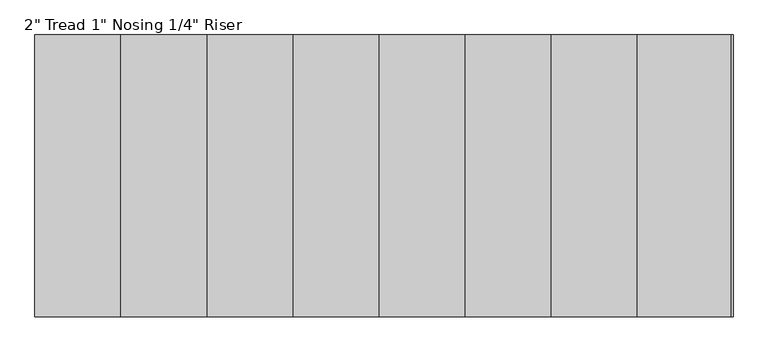
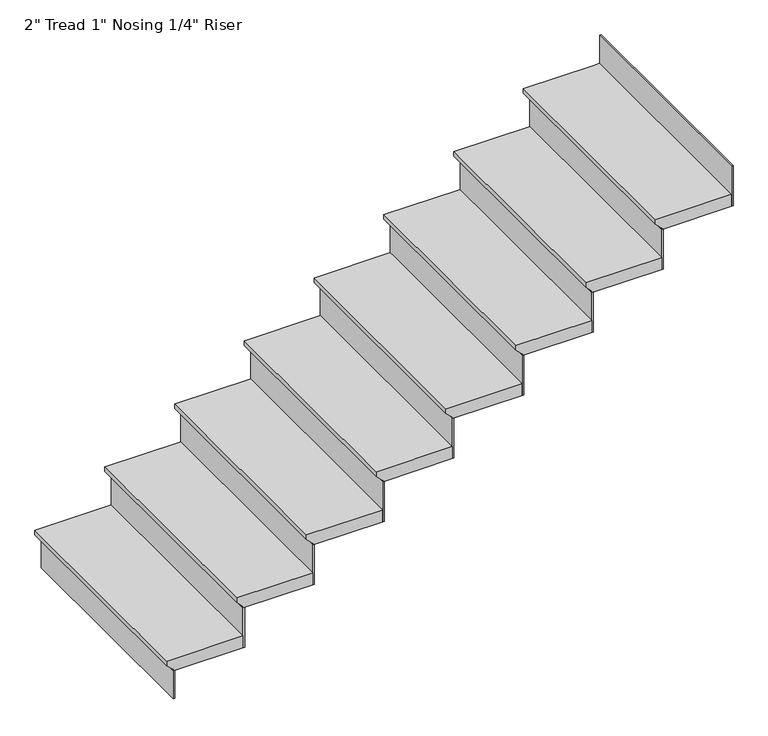
"""IFC4 building model written with IfcOpenShell, lengths in millimetres: stair flight geometry."""

from ifc_helpers import new_model, si_unit, origin, place, context, project, spatial, faceted_brep, source, transform, mapped, element, save


def stair_flight_35773103(model_context):
    return source(origin(), model_context, "Body", "Brep", [
        faceted_brep([(-8529.8389568, 3195.5342758, 150.2833333), (-8529.8389568, 3195.5342758, 169.3333333), (-8529.8389568, 4109.9342758, 169.3333333), (-8529.8389568, 4109.9342758, 150.2833333), (-8504.4389568, 3195.5342758, 124.8833333), (-8504.4389568, 4109.9342758, 124.8833333), (-8225.0389568, 3195.5342758, 169.3333333), (-8225.0389568, 4109.9342758, 169.3333333), (-8504.4389568, 4109.9342758, 118.5333333), (-8225.0389568, 4109.9342758, 118.5333333), (-8225.0389568, 3195.5342758, 118.5333333), (-8504.4389568, 3195.5342758, 118.5333333)], [[[0, 1, 2, 3]], [[4, 0, 3, 5]], [[2, 1, 6, 7]], [[8, 9, 10, 11]], [[2, 7, 9, 8, 5, 3]], [[8, 11, 4, 5]], [[6, 1, 0, 4, 11, 10]], [[7, 6, 10, 9]]]),
        faceted_brep([(-8504.4389568, 3195.5342758, 118.5333333), (-8504.4389568, 3195.5342758, 0.0), (-8498.0889568, 3195.5342758, 0.0), (-8498.0889568, 3195.5342758, 118.5333333), (-8504.4389568, 4109.9342758, 118.5333333), (-8498.0889568, 4109.9342758, 118.5333333), (-8498.0889568, 4109.9342758, 0.0), (-8504.4389568, 4109.9342758, 0.0)], [[[0, 1, 2, 3]], [[4, 5, 6, 7]], [[1, 0, 4, 7]], [[2, 1, 7, 6]], [[3, 2, 6, 5]], [[0, 3, 5, 4]]]),
        faceted_brep([(-8225.0389568, 3195.5342758, 287.8666667), (-8225.0389568, 3195.5342758, 118.5333333), (-8218.6889568, 3195.5342758, 118.5333333), (-8218.6889568, 3195.5342758, 287.8666667), (-8225.0389568, 4109.9342758, 287.8666667), (-8218.6889568, 4109.9342758, 287.8666667), (-8218.6889568, 4109.9342758, 118.5333333), (-8225.0389568, 4109.9342758, 118.5333333)], [[[0, 1, 2, 3]], [[4, 5, 6, 7]], [[1, 0, 4, 7]], [[2, 1, 7, 6]], [[3, 2, 6, 5]], [[0, 3, 5, 4]]]),
        faceted_brep([(-8250.4389568, 4109.9342758, 338.6666667), (-8250.4389568, 3195.5342758, 338.6666667), (-7945.6389568, 3195.5342758, 338.6666667), (-7945.6389568, 4109.9342758, 338.6666667), (-8225.0389568, 4109.9342758, 287.8666667), (-7945.6389568, 4109.9342758, 287.8666667), (-7945.6389568, 3195.5342758, 287.8666667), (-8225.0389568, 3195.5342758, 287.8666667), (-8225.0389568, 4109.9342758, 294.2166667), (-8250.4389568, 4109.9342758, 319.6166667), (-8225.0389568, 3195.5342758, 294.2166667), (-8250.4389568, 3195.5342758, 319.6166667)], [[[0, 1, 2, 3]], [[4, 5, 6, 7]], [[0, 3, 5, 4, 8, 9]], [[4, 7, 10, 8]], [[2, 1, 11, 10, 7, 6]], [[3, 2, 6, 5]], [[11, 1, 0, 9]], [[10, 11, 9, 8]]]),
        faceted_brep([(-7945.6389568, 3195.5342758, 457.2), (-7945.6389568, 3195.5342758, 287.8666667), (-7939.2889568, 3195.5342758, 287.8666667), (-7939.2889568, 3195.5342758, 457.2), (-7945.6389568, 4109.9342758, 457.2), (-7939.2889568, 4109.9342758, 457.2), (-7939.2889568, 4109.9342758, 287.8666667), (-7945.6389568, 4109.9342758, 287.8666667)], [[[0, 1, 2, 3]], [[4, 5, 6, 7]], [[1, 0, 4, 7]], [[2, 1, 7, 6]], [[3, 2, 6, 5]], [[0, 3, 5, 4]]]),
        faceted_brep([(-7971.0389568, 4109.9342758, 508.0), (-7971.0389568, 3195.5342758, 508.0), (-7666.2389568, 3195.5342758, 508.0), (-7666.2389568, 4109.9342758, 508.0), (-7945.6389568, 4109.9342758, 457.2), (-7666.2389568, 4109.9342758, 457.2), (-7666.2389568, 3195.5342758, 457.2), (-7945.6389568, 3195.5342758, 457.2), (-7945.6389568, 4109.9342758, 463.55), (-7971.0389568, 4109.9342758, 488.95), (-7945.6389568, 3195.5342758, 463.55), (-7971.0389568, 3195.5342758, 488.95)], [[[0, 1, 2, 3]], [[4, 5, 6, 7]], [[0, 3, 5, 4, 8, 9]], [[4, 7, 10, 8]], [[2, 1, 11, 10, 7, 6]], [[3, 2, 6, 5]], [[11, 1, 0, 9]], [[10, 11, 9, 8]]]),
        faceted_brep([(-7666.2389568, 3195.5342758, 626.5333333), (-7666.2389568, 3195.5342758, 457.2), (-7659.8889568, 3195.5342758, 457.2), (-7659.8889568, 3195.5342758, 626.5333333), (-7666.2389568, 4109.9342758, 626.5333333), (-7659.8889568, 4109.9342758, 626.5333333), (-7659.8889568, 4109.9342758, 457.2), (-7666.2389568, 4109.9342758, 457.2)], [[[0, 1, 2, 3]], [[4, 5, 6, 7]], [[1, 0, 4, 7]], [[2, 1, 7, 6]], [[3, 2, 6, 5]], [[0, 3, 5, 4]]]),
        faceted_brep([(-7691.6389568, 4109.9342758, 677.3333333), (-7691.6389568, 3195.5342758, 677.3333333), (-7386.8389568, 3195.5342758, 677.3333333), (-7386.8389568, 4109.9342758, 677.3333333), (-7666.2389568, 4109.9342758, 626.5333333), (-7386.8389568, 4109.9342758, 626.5333333), (-7386.8389568, 3195.5342758, 626.5333333), (-7666.2389568, 3195.5342758, 626.5333333), (-7666.2389568, 4109.9342758, 632.8833333), (-7691.6389568, 4109.9342758, 658.2833333), (-7666.2389568, 3195.5342758, 632.8833333), (-7691.6389568, 3195.5342758, 658.2833333)], [[[0, 1, 2, 3]], [[4, 5, 6, 7]], [[0, 3, 5, 4, 8, 9]], [[4, 7, 10, 8]], [[2, 1, 11, 10, 7, 6]], [[3, 2, 6, 5]], [[11, 1, 0, 9]], [[10, 11, 9, 8]]]),
        faceted_brep([(-7386.8389568, 3195.5342758, 795.8666667), (-7386.8389568, 3195.5342758, 626.5333333), (-7380.4889568, 3195.5342758, 626.5333333), (-7380.4889568, 3195.5342758, 795.8666667), (-7386.8389568, 4109.9342758, 795.8666667), (-7380.4889568, 4109.9342758, 795.8666667), (-7380.4889568, 4109.9342758, 626.5333333), (-7386.8389568, 4109.9342758, 626.5333333)], [[[0, 1, 2, 3]], [[4, 5, 6, 7]], [[1, 0, 4, 7]], [[2, 1, 7, 6]], [[3, 2, 6, 5]], [[0, 3, 5, 4]]]),
        faceted_brep([(-7412.2389568, 4109.9342758, 846.6666667), (-7412.2389568, 3195.5342758, 846.6666667), (-7107.4389568, 3195.5342758, 846.6666667), (-7107.4389568, 4109.9342758, 846.6666667), (-7386.8389568, 4109.9342758, 795.8666667), (-7107.4389568, 4109.9342758, 795.8666667), (-7107.4389568, 3195.5342758, 795.8666667), (-7386.8389568, 3195.5342758, 795.8666667), (-7386.8389568, 4109.9342758, 802.2166667), (-7412.2389568, 4109.9342758, 827.6166667), (-7386.8389568, 3195.5342758, 802.2166667), (-7412.2389568, 3195.5342758, 827.6166667)], [[[0, 1, 2, 3]], [[4, 5, 6, 7]], [[0, 3, 5, 4, 8, 9]], [[4, 7, 10, 8]], [[2, 1, 11, 10, 7, 6]], [[3, 2, 6, 5]], [[11, 1, 0, 9]], [[10, 11, 9, 8]]]),
        faceted_brep([(-7107.4389568, 3195.5342758, 965.2), (-7107.4389568, 3195.5342758, 795.8666667), (-7101.0889568, 3195.5342758, 795.8666667), (-7101.0889568, 3195.5342758, 965.2), (-7107.4389568, 4109.9342758, 965.2), (-7101.0889568, 4109.9342758, 965.2), (-7101.0889568, 4109.9342758, 795.8666667), (-7107.4389568, 4109.9342758, 795.8666667)], [[[0, 1, 2, 3]], [[4, 5, 6, 7]], [[1, 0, 4, 7]], [[2, 1, 7, 6]], [[3, 2, 6, 5]], [[0, 3, 5, 4]]]),
        faceted_brep([(-7132.8389568, 4109.9342758, 1016.0), (-7132.8389568, 3195.5342758, 1016.0), (-6828.0389568, 3195.5342758, 1016.0), (-6828.0389568, 4109.9342758, 1016.0), (-7107.4389568, 4109.9342758, 965.2), (-6828.0389568, 4109.9342758, 965.2), (-6828.0389568, 3195.5342758, 965.2), (-7107.4389568, 3195.5342758, 965.2), (-7107.4389568, 4109.9342758, 971.55), (-7132.8389568, 4109.9342758, 996.95), (-7107.4389568, 3195.5342758, 971.55), (-7132.8389568, 3195.5342758, 996.95)], [[[0, 1, 2, 3]], [[4, 5, 6, 7]], [[0, 3, 5, 4, 8, 9]], [[4, 7, 10, 8]], [[2, 1, 11, 10, 7, 6]], [[3, 2, 6, 5]], [[11, 1, 0, 9]], [[10, 11, 9, 8]]]),
        faceted_brep([(-6828.0389568, 3195.5342758, 1134.5333333), (-6828.0389568, 3195.5342758, 965.2), (-6821.6889568, 3195.5342758, 965.2), (-6821.6889568, 3195.5342758, 1134.5333333), (-6828.0389568, 4109.9342758, 1134.5333333), (-6821.6889568, 4109.9342758, 1134.5333333), (-6821.6889568, 4109.9342758, 965.2), (-6828.0389568, 4109.9342758, 965.2)], [[[0, 1, 2, 3]], [[4, 5, 6, 7]], [[1, 0, 4, 7]], [[2, 1, 7, 6]], [[3, 2, 6, 5]], [[0, 3, 5, 4]]]),
        faceted_brep([(-6853.4389568, 4109.9342758, 1185.3333333), (-6853.4389568, 3195.5342758, 1185.3333333), (-6548.6389568, 3195.5342758, 1185.3333333), (-6548.6389568, 4109.9342758, 1185.3333333), (-6828.0389568, 4109.9342758, 1134.5333333), (-6548.6389568, 4109.9342758, 1134.5333333), (-6548.6389568, 3195.5342758, 1134.5333333), (-6828.0389568, 3195.5342758, 1134.5333333), (-6828.0389568, 4109.9342758, 1140.8833333), (-6853.4389568, 4109.9342758, 1166.2833333), (-6828.0389568, 3195.5342758, 1140.8833333), (-6853.4389568, 3195.5342758, 1166.2833333)], [[[0, 1, 2, 3]], [[4, 5, 6, 7]], [[0, 3, 5, 4, 8, 9]], [[4, 7, 10, 8]], [[2, 1, 11, 10, 7, 6]], [[3, 2, 6, 5]], [[11, 1, 0, 9]], [[10, 11, 9, 8]]]),
        faceted_brep([(-6269.2389568, 3195.5342758, 1473.2), (-6269.2389568, 3195.5342758, 1303.8666667), (-6262.8889568, 3195.5342758, 1303.8666667), (-6262.8889568, 3195.5342758, 1473.2), (-6269.2389568, 4109.9342758, 1473.2), (-6262.8889568, 4109.9342758, 1473.2), (-6262.8889568, 4109.9342758, 1303.8666667), (-6269.2389568, 4109.9342758, 1303.8666667)], [[[0, 1, 2, 3]], [[4, 5, 6, 7]], [[1, 0, 4, 7]], [[2, 1, 7, 6]], [[3, 2, 6, 5]], [[0, 3, 5, 4]]]),
        faceted_brep([(-6548.6389568, 3195.5342758, 1303.8666667), (-6548.6389568, 3195.5342758, 1134.5333333), (-6542.2889568, 3195.5342758, 1134.5333333), (-6542.2889568, 3195.5342758, 1303.8666667), (-6548.6389568, 4109.9342758, 1303.8666667), (-6542.2889568, 4109.9342758, 1303.8666667), (-6542.2889568, 4109.9342758, 1134.5333333), (-6548.6389568, 4109.9342758, 1134.5333333)], [[[0, 1, 2, 3]], [[4, 5, 6, 7]], [[1, 0, 4, 7]], [[2, 1, 7, 6]], [[3, 2, 6, 5]], [[0, 3, 5, 4]]]),
        faceted_brep([(-6269.2389568, 4109.9342758, 1354.6666667), (-6294.6389568, 4109.9342758, 1354.6666667), (-6574.0389568, 4109.9342758, 1354.6666667), (-6574.0389568, 3195.5342758, 1354.6666667), (-6269.2389568, 3195.5342758, 1354.6666667), (-6294.6389568, 4109.9342758, 1303.8666667), (-6269.2389568, 4109.9342758, 1303.8666667), (-6269.2389568, 3195.5342758, 1303.8666667), (-6548.6389568, 3195.5342758, 1303.8666667), (-6548.6389568, 4109.9342758, 1303.8666667), (-6548.6389568, 4109.9342758, 1310.2166667), (-6574.0389568, 4109.9342758, 1335.6166667), (-6548.6389568, 3195.5342758, 1310.2166667), (-6574.0389568, 3195.5342758, 1335.6166667)], [[[0, 1, 2, 3, 4]], [[5, 6, 7, 8, 9]], [[1, 0, 6, 5]], [[2, 1, 5, 9, 10, 11]], [[9, 8, 12, 10]], [[4, 3, 13, 12, 8, 7]], [[0, 4, 7, 6]], [[13, 3, 2, 11]], [[12, 13, 11, 10]]]),
    ])


if __name__ == "__main__":
    model = new_model("IFC4")
    model_context = context("Model", 3, world=origin())
    ifc_project = project(units=[si_unit("LENGTHUNIT", "METRE", prefix="MILLI")], contexts=[model_context])
    site = spatial("IfcSite", under=ifc_project)
    building = spatial("IfcBuilding", under=site)
    placement = place(None, origin())
    stair_flight_shape = stair_flight_35773103(model_context)
    element("IfcStairFlight", 1, ObjectType="2\" Tread 1\" Nosing 1/4\" Riser", at=placement, inside=building, context=model_context, shape_type="MappedRepresentation", body=[
        mapped(stair_flight_shape, transform((0.0, 0.0, 0.0), x_axis=(1.0, 0.0, 0.0), y_axis=(0.0, 1.0, 0.0), z_axis=(0.0, 0.0, 1.0))),
    ])
    save(model, "model.ifc")
